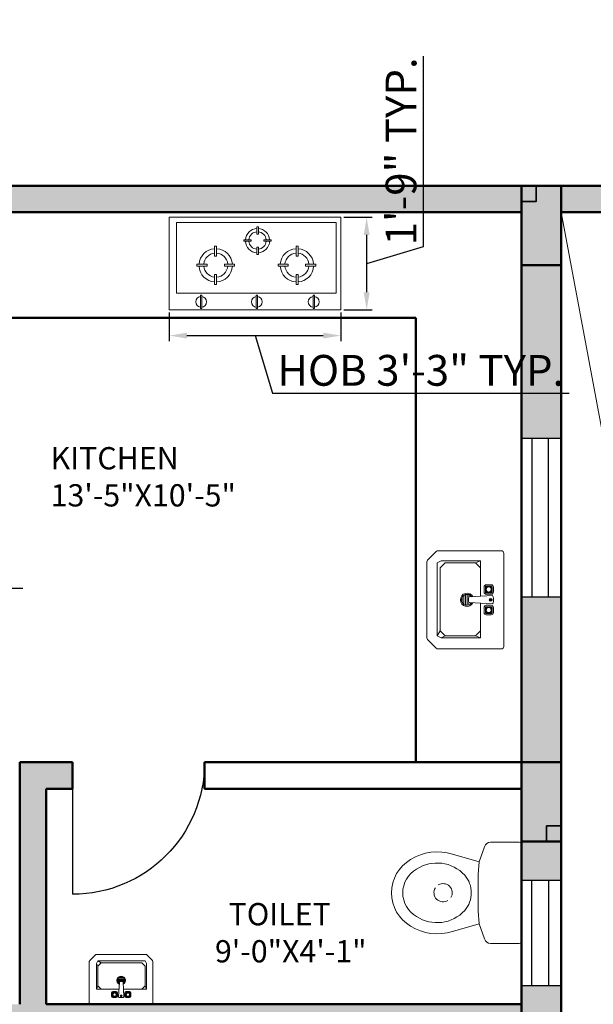
# Model space of a CAD drawing. Units: inches. Extents: x -7 to 1228, y -146 to 1091.
# Tile 25 of 88: x 433 to 563, y 307 to 531. Entities that reach past the tile are written whole.
import ezdxf

# ---------------------------------------------------------------- set-up
doc = ezdxf.new("R2010")
doc.units = ezdxf.units.IN
for name, color, linetype, lineweight in [('A-ANNO-DIMS', 2, 'Continuous', 18), ('A-AREA-IDEN', 7, 'Continuous', 18), ('A-COLS', 6, 'Continuous', 35), ('A-DOOR', 4, 'Continuous', 25), ('A-FLOR-FIXT', 8, 'Continuous', 18), ('A-FLOR-VOID', 7, 'Continuous', 18), ('A-FURN', 8, 'Continuous', 18), ('A-GLAZ', 175, 'Continuous', 25), ('A-WALL', 7, 'Continuous', 50), ('A-WALL-PATT', 251, 'Continuous', 13)]:
    doc.layers.add(name, color=color, linetype=linetype, lineweight=lineweight)
doc.styles.get("Standard").update_dxf_attribs({"font": 'arial.ttf'})
doc.dimstyles.new('ISO-25', dxfattribs={"dimtxt": 7, "dimasz": 4, "dimexe": 1.25, "dimexo": 0.625, "dimtad": 1, "dimdec": 1, "dimlunit": 3, "dimtxsty": 'Standard', "dimcen": 2.5, "dimadec": 0, "dimazin": 0, "dimtfac": 1, "dimtdec": 1, "dimtmove": 1, "dimatfit": 3, "dimfxl": 1, "dimarcsym": 0})

# ---------------------------------------------------------------- blocks, each defined once
blk = doc.blocks.new('A$C72243D80')
at = {"ltscale": 1000}
for p, q in [((0, 0), (0, 384.2)), ((0, 384.2), (712, 384.2)), ((712, 384.2), (712, 0)), ((29.5, 68.9), (29.5, 363.2)), ((29.5, 363.2), (692.7, 363.2)), ((363.5, 314.5), (363.5, 345.1)), ((363.5, 345.1), (369.5, 345.1)), ((369.5, 345.1), (369.5, 314.5)), ((692.7, 363.2), (692.7, 68.9)), ((309.4, 291), (340, 291)), ((309.4, 285), (309.4, 291)), ((340, 291), (340, 285)), ((369.5, 314.5), (363.5, 314.5)), ((392.3, 291), (392.3, 285)), ((422.9, 291), (392.3, 291)), ((422.9, 285), (422.9, 291)), ((188.1, 264.2), (188.1, 222.1)), ((196.4, 264.2), (188.1, 264.2)), ((196.4, 222.1), (196.4, 264.2)), ((340, 285), (309.4, 285)), ((363.5, 260), (363.5, 229.4)), ((369.5, 260), (363.5, 260)), ((369.5, 229.4), (369.5, 260)), ((392.3, 285), (422.9, 285)), ((525.9, 222.1), (525.9, 264.2)), ((525.9, 264.2), (534.1, 264.2)), ((534.1, 264.2), (534.1, 222.1)), ((188.1, 222.1), (196.4, 222.1)), ((363.5, 229.4), (369.5, 229.4)), ((534.1, 222.1), (525.9, 222.1)), ((114.7, 189.8), (156.8, 189.8)), ((114.7, 181.6), (114.7, 189.8)), ((156.8, 181.6), (114.7, 181.6)), ((156.8, 189.8), (156.8, 181.6)), ((228.6, 189.8), (228.6, 181.6)), ((270.7, 189.8), (228.6, 189.8)), ((228.6, 181.6), (270.7, 181.6)), ((270.7, 181.6), (270.7, 189.8)), ((451.5, 189.8), (493.6, 189.8)), ((451.5, 181.6), (451.5, 189.8)), ((493.6, 181.6), (451.5, 181.6)), ((493.6, 189.8), (493.6, 181.6)), ((565.5, 189.8), (565.5, 181.6)), ((607.6, 189.8), (565.5, 189.8)), ((565.5, 181.6), (607.6, 181.6)), ((607.6, 181.6), (607.6, 189.8)), ((188.1, 147.2), (196.4, 147.2)), ((188.1, 105.1), (188.1, 147.2)), ((196.4, 147.2), (196.4, 105.1)), ((525.9, 147.2), (525.9, 105.1)), ((534.1, 147.2), (525.9, 147.2)), ((534.1, 105.1), (534.1, 147.2)), ((196.4, 105.1), (188.1, 105.1)), ((525.9, 105.1), (534.1, 105.1)), ((692.7, 68.9), (29.5, 68.9)), ((129.6, 61.1), (129.6, 5)), ((134.4, 61.1), (129.6, 61.1)), ((134.4, 5), (134.4, 61.1)), ((360.9, 5), (360.9, 61.1)), ((360.9, 61.1), (365.7, 61.1)), ((365.7, 61.1), (365.7, 5)), ((597, 5), (597, 61.1)), ((597, 61.1), (601.8, 61.1)), ((601.8, 61.1), (601.8, 5)), ((712, 0), (0, 0)), ((129.6, 5), (134.4, 5)), ((365.7, 5), (360.9, 5)), ((601.8, 5), (597, 5))]:
    blk.add_line(p, q, dxfattribs=at)
for centre, radius, start, end in [((366.2, 287.2), 50.3, 93.0344, 175.7271), ((366.2, 287.2), 50.3, 4.2729, 86.1838), ((366.1, 287.8), 36.3, 94.0374, 175.0142), ((366.1, 287.8), 36.3, 4.9858, 84.5356), ((192.7, 184.7), 69.2, 93.8162, 175.7271), ((192.7, 184.7), 69.2, 4.2729, 86.9656), ((366.2, 287.2), 50.3, 182.5783, 266.9656), ((366.1, 287.8), 36.3, 184.5153, 265.9626), ((366.1, 287.8), 36.3, 275.4644, 355.4847), ((366.2, 287.2), 50.3, 273.8162, 357.4217), ((529.5, 184.7), 69.2, 93.0344, 175.7271), ((529.5, 184.7), 69.2, 4.2729, 86.1838), ((192.9, 185.5), 49.9, 95.4644, 175.0142), ((192.9, 185.5), 49.9, 4.9858, 85.9626), ((529.4, 185.5), 49.9, 94.0374, 175.0142), ((529.4, 185.5), 49.9, 4.9858, 84.5356), ((192.7, 184.7), 69.2, 182.5783, 266.1838), ((192.9, 185.5), 49.9, 184.5153, 264.5356), ((192.9, 185.5), 49.9, 274.0374, 355.4847), ((192.7, 184.7), 69.2, 273.0344, 357.4217), ((529.5, 184.7), 69.2, 182.5783, 266.9656), ((529.4, 185.5), 49.9, 184.5153, 265.9626), ((529.5, 184.7), 69.2, 273.8162, 357.4217), ((529.4, 185.5), 49.9, 275.4644, 355.4847), ((132.3, 33.2), 22.5, 96.7453, 263.2547), ((132.3, 33.2), 22.5, 275.4789, 84.5211), ((363.1, 33.2), 22.5, 95.4789, 264.5211), ((363.1, 33.2), 22.5, 276.7453, 83.2547), ((599.2, 33.2), 22.5, 95.4789, 264.5211), ((599.2, 33.2), 22.5, 276.7453, 83.2547)]:
    blk.add_arc(centre, radius, start, end, dxfattribs=at)
blk = doc.blocks.new('A$C4CB854FF')
for p, q in [((0, 0.3675), (0, 0.0552)), ((0.4725, 0.38), (0.0125, 0.38)), ((0.485, 0.0552), (0.485, 0.3675)), ((0.1677, 0.2932), (0.1677, 0.318)), ((0.1745, 0.2919), (0.1745, 0.3194)), ((0.1773, 0.3221), (0.2048, 0.3221)), ((0.1787, 0.329), (0.2034, 0.329)), ((0.2075, 0.3194), (0.2075, 0.2919)), ((0.2144, 0.318), (0.2144, 0.2932)), ((0.2279, 0.2104), (0.2213, 0.3235)), ((0.2337, 0.329), (0.2502, 0.329)), ((0.2625, 0.3235), (0.256, 0.2104)), ((0.2694, 0.318), (0.2694, 0.2932)), ((0.2763, 0.3194), (0.2763, 0.2919)), ((0.3065, 0.3221), (0.279, 0.3221)), ((0.3052, 0.329), (0.2804, 0.329)), ((0.3093, 0.2919), (0.3093, 0.3194)), ((0.3162, 0.2932), (0.3162, 0.318)), ((0.05, 0.265), (0.2247, 0.265)), ((0.06, 0.24), (0.05, 0.265)), ((0.05, 0.07), (0.05, 0.265)), ((0.085, 0.265), (0.06, 0.24)), ((0.2048, 0.2891), (0.1773, 0.2891)), ((0.2034, 0.2822), (0.1787, 0.2822)), ((0.2591, 0.265), (0.43, 0.265)), ((0.279, 0.2891), (0.3065, 0.2891)), ((0.2804, 0.2822), (0.3052, 0.2822)), ((0.395, 0.265), (0.42, 0.24)), ((0.42, 0.24), (0.43, 0.265)), ((0.43, 0.07), (0.43, 0.265)), ((0.06, 0.24), (0.06, 0.09)), ((0.2152, 0.1984), (0.2694, 0.1984)), ((0.2297, 0.2066), (0.2165, 0.2066)), ((0.2272, 0.2149), (0.2208, 0.2149)), ((0.2505, 0.2052), (0.2334, 0.2052)), ((0.2681, 0.2066), (0.2541, 0.2066)), ((0.2638, 0.2149), (0.2566, 0.2149)), ((0.42, 0.24), (0.42, 0.09)), ((0.2681, 0.1901), (0.2165, 0.1901)), ((0.2638, 0.1819), (0.2208, 0.1819)), ((0.2533, 0.1736), (0.2313, 0.1736)), ((0.05, 0.07), (0.06, 0.05)), ((0.06, 0.09), (0.085, 0.065)), ((0.42, 0.05), (0.06, 0.05)), ((0.085, 0.065), (0.395, 0.065)), ((0.42, 0.09), (0.395, 0.065)), ((0.395, 0.065), (0.42, 0.05)), ((0.42, 0.09), (0.43, 0.07)), ((0.43, 0.07), (0.42, 0.05)), ((0.0037, 0.0463), (0.0463, 0.0037)), ((0.4387, 0.0037), (0.4813, 0.0463)), ((0.0552, 0), (0.4298, 0))]:
    blk.add_line(p, q)
for centre, radius in [((0.191, 0.3056), 0.0165), ((0.191, 0.3056), 0.0127), ((0.2419, 0.3152), 0.00688), ((0.2419, 0.3152), 0.00344), ((0.2928, 0.3056), 0.0165), ((0.2928, 0.3056), 0.0127)]:
    blk.add_circle(centre, radius)
for centre, radius, start, end in [((0.0125, 0.3675), 0.0125, 90, 180), ((0.4725, 0.3675), 0.0125, 0, 90), ((0.1787, 0.318), 0.011, 90, 180), ((0.1787, 0.2932), 0.011, 180, 270), ((0.1773, 0.3194), 0.00275, 90, 180), ((0.2034, 0.318), 0.011, 0, 90), ((0.2034, 0.2932), 0.011, 270, 0), ((0.2048, 0.3194), 0.00275, 360, 90), ((0.2329, 0.314), 0.015, 87.1975, 140.7274), ((0.2509, 0.314), 0.015, 39.2726, 92.8025), ((0.2804, 0.318), 0.011, 90, 180), ((0.2804, 0.2932), 0.011, 180, 270), ((0.279, 0.3194), 0.00275, 90, 180), ((0.3052, 0.318), 0.011, 0, 90), ((0.3052, 0.2932), 0.011, 270, 360), ((0.3065, 0.3194), 0.00275, 360, 90), ((0.1773, 0.2919), 0.00275, 180, 270), ((0.2048, 0.2919), 0.00275, 270, 0), ((0.279, 0.2919), 0.00275, 180, 270), ((0.3065, 0.2919), 0.00275, 270, 0), ((0.2423, 0.1984), 0.033, 118.6883, 62.8686), ((0.2423, 0.1984), 0.0271, 124.7758, 57.2247), ((0.2334, 0.2107), 0.0055, 183.3274, 270), ((0.2505, 0.2107), 0.0055, 270, 356.6726), ((0.0125, 0.0552), 0.0125, 180, 225), ((0.4725, 0.0552), 0.0125, 315, 0), ((0.0552, 0.0125), 0.0125, 225, 270), ((0.4298, 0.0125), 0.0125, 270, 315)]:
    blk.add_arc(centre, radius, start, end)
blk = doc.blocks.new('A$C7B5C7CD4')
at = {"ltscale": 20}
for p, q in [((0.243, 0.625), (0.011, 0.625)), ((0.243, 0.625), (0.475, 0.625)), ((0, 0.614), (0, 0.4765)), ((0.486, 0.614), (0.486, 0.4765)), ((0.0212, 0.4467), (0.0946, 0.4214)), ((0.4648, 0.4467), (0.3914, 0.4214)), ((0.0946, 0.4214), (0.0576, 0.293)), ((0.0946, 0.4214), (0.1544, 0.4173)), ((0.3316, 0.4173), (0.1544, 0.4173)), ((0.3914, 0.4214), (0.3316, 0.4173)), ((0.3914, 0.4214), (0.4284, 0.293))]:
    blk.add_line(p, q, dxfattribs=at)
for centre, radius, start, end in [((0.011, 0.614), 0.011, 90, 180), ((0.475, 0.614), 0.011, 0, 90), ((0.0315, 0.4765), 0.0315, 180, 251), ((0.4545, 0.4765), 0.0315, 289, 0), ((0.24, 0.2602), 0.123, 88.6158, 131.7414), ((0.246, 0.2602), 0.123, 48.2586, 91.3842), ((0.2796, 0.219), 0.18, 132.4207, 213.289), ((0.2064, 0.219), 0.18, 326.711, 47.5793), ((0.2796, 0.219), 0.234, 161.5846, 212.8753), ((0.2064, 0.219), 0.234, 327.1247, 18.4154), ((0.243, 0.185), 0.131, 209.6292, 270), ((0.243, 0.185), 0.131, 270, 330.3708), ((0.243, 0.185), 0.185, 210.1745, 270), ((0.243, 0.185), 0.185, 270, 329.8255)]:
    blk.add_arc(centre, radius, start, end, dxfattribs=at)
for start, end in [(58.1785, 211.8215), (238.1785, 31.8215)]:
    blk.add_arc((0.2426, 0.2481), 0.0439, start, end)
blk = doc.blocks.new('WIN-36')
for p, q in [((0, 36), (0, 0)), ((9, 36), (0, 36)), ((2.34, 36), (2.34, 0)), ((6.14, 0), (6.14, 36)), ((9, 0), (9, 36)), ((0, 0), (9, 0)), ((2.34, 0), (6.14, 0))]:
    blk.add_line(p, q)
blk = doc.blocks.new('WIN-24')
for p, q in [((0, 0), (0, 24)), ((0, 24), (9, 24)), ((2.34, 0), (2.34, 24)), ((2.34, 24), (6.14, 24)), ((6.14, 24), (6.14, 0)), ((9, 24), (9, 0)), ((9, 0), (0, 0))]:
    blk.add_line(p, q)
blk = doc.blocks.new('DOOR-750')
blk.add_line((30, 30), (30, 0))
blk.add_arc((30, 30), 30, 180, 270)
blk = doc.blocks.new('*D34')
at = {"layer": 'A-ANNO-DIMS', "color": 0, "lineweight": -2, "transparency": 16777216}
for p, q in [((466.98, 464.2), (466.98, 457.73)), ((505.97, 464.2), (505.97, 457.73)), ((470.98, 458.98), (501.97, 458.98)), ((486.48, 458.98), (490.4, 445.92)), ((490.4, 445.92), (557.85, 445.92))]:
    blk.add_line(p, q, dxfattribs=at)
at = {"layer": 'A-ANNO-DIMS', "color": 0, "transparency": 16777216}
for points in [[(470.98, 459.64), (470.98, 458.31), (466.98, 458.98)], [(501.97, 459.64), (501.97, 458.31), (505.97, 458.98)]]:
    blk.add_solid(points, dxfattribs=at)
at = {"layer": 'Defpoints', "color": 0, "transparency": 16777216}
for p in [(466.98, 464.83), (505.97, 464.83), (505.97, 458.98)]:
    blk.add_point(p, dxfattribs=at)
at = {"layer": 'A-ANNO-DIMS', "color": 0, "transparency": 16777216, "insert": (524.12, 450.17), "char_height": 7, "attachment_point": 5}
blk.add_mtext('HOB 3\'-3" TYP.', dxfattribs=at)
blk = doc.blocks.new('*D35')
at = {"layer": 'A-ANNO-DIMS', "color": 0, "lineweight": -2, "transparency": 16777216}
for p, q in [((524.73, 479.22), (524.73, 522.48)), ((506.6, 485.86), (513.07, 485.86)), ((511.82, 468.83), (511.82, 481.86)), ((511.82, 475.34), (524.73, 479.22)), ((506.6, 464.83), (513.07, 464.83))]:
    blk.add_line(p, q, dxfattribs=at)
at = {"layer": 'A-ANNO-DIMS', "color": 0, "transparency": 16777216}
for points in [[(511.15, 481.86), (512.49, 481.86), (511.82, 485.86)], [(511.15, 468.83), (512.49, 468.83), (511.82, 464.83)]]:
    blk.add_solid(points, dxfattribs=at)
at = {"layer": 'Defpoints', "color": 0, "transparency": 16777216}
for p in [(505.97, 485.86), (511.82, 485.86), (505.97, 464.83)]:
    blk.add_point(p, dxfattribs=at)
at = {"layer": 'A-ANNO-DIMS', "color": 0, "transparency": 16777216, "insert": (520.53, 500.85), "char_height": 7, "attachment_point": 5, "rotation": 90}
blk.add_mtext('1\'-9" TYP.', dxfattribs=at)
blk = doc.blocks.new('*D40')
at = {"layer": 'A-ANNO-DIMS', "color": 0, "lineweight": -2, "transparency": 16777216}
for p, q in [((301.32, 424.02), (301.32, 413.35)), ((368.31, 424.02), (368.31, 413.35)), ((305.32, 414.6), (364.31, 414.6)), ((334.82, 414.6), (338.73, 401.55)), ((338.73, 401.55), (433.69, 401.55))]:
    blk.add_line(p, q, dxfattribs=at)
at = {"layer": 'A-ANNO-DIMS', "color": 0, "transparency": 16777216}
for points in [[(305.32, 415.26), (305.32, 413.93), (301.32, 414.6)], [(364.31, 415.26), (364.31, 413.93), (368.31, 414.6)]]:
    blk.add_solid(points, dxfattribs=at)
at = {"layer": 'Defpoints', "color": 0, "transparency": 16777216}
for p in [(301.32, 424.65), (368.31, 424.65), (368.31, 414.6)]:
    blk.add_point(p, dxfattribs=at)
at = {"layer": 'A-ANNO-DIMS', "color": 0, "transparency": 16777216, "insert": (386.21, 405.79), "char_height": 7, "attachment_point": 5}
blk.add_mtext('SOFA SET 5\'-7" TYP.', dxfattribs=at)

msp = doc.modelspace()

# ---------------------------------------------------------------- hatches: boundary and pattern name
at = {"layer": 'A-COLS'}
h = msp.add_hatch(color=256, dxfattribs=at)
h.dxf.hatch_style = 1
h.paths.add_polyline_path([(547, 475), (556, 475), (556, 493), (550.29, 493), (550.29, 489.45), (547, 489.45)])
h = msp.add_hatch(color=256, dxfattribs=at)
h.dxf.hatch_style = 1
h.paths.add_polyline_path([(550.29, 489.45), (550.29, 493), (547, 493), (547, 489.45)])
h = msp.add_hatch(color=256, dxfattribs=at)
h.dxf.hatch_style = 1
h.paths.add_polyline_path([(556, 362), (547, 362), (547, 344), (552.71, 344), (552.71, 347.55), (556, 347.55)])
h = msp.add_hatch(color=256, dxfattribs=at)
h.dxf.hatch_style = 1
h.paths.add_polyline_path([(552.71, 347.55), (552.71, 344), (556, 344), (556, 347.55)])
at = {"layer": 'A-WALL-PATT'}
h = msp.add_hatch(color=256, dxfattribs=at)
h.dxf.hatch_style = 1
h.paths.add_polyline_path([(69, 568), (60, 568), (60, 493), (63.29, 493), (69, 493)])
h.paths.add_polyline_path([(69, 662.41), (60, 662.41), (60, 586), (69, 586)], flags=17)
h.paths.add_polyline_path([(69, 723), (184, 723), (184, 734), (179, 734), (179, 728), (69, 728), (69, 741.62), (60, 741.62), (60, 698.41), (69, 698.41)], flags=17)
h.paths.add_polyline_path([(69, 782), (231, 782), (231, 728), (231, 723), (231, 586), (236, 586), (236, 787), (69, 787), (69, 800.13), (60, 800.13), (60, 765.62), (69, 765.62)])
h.paths.add_polyline_path([(184, 842), (189, 842), (189, 848), (173, 848), (173, 842), (179, 842), (179, 787), (184, 787)])
h.paths.add_polyline_path([(118.22, 69), (69, 69), (69, 60), (118.22, 60)])
h.paths.add_polyline_path([(227, 69), (154.22, 69), (154.22, 60), (227, 60)])
h.paths.add_polyline_path([(236, 60), (232.71, 60), (227, 60), (227, 36), (236, 36)])
h.paths.add_polyline_path([(389, 60), (380, 60), (380, 36), (389, 36)])
h.paths.add_polyline_path([(384, 181), (380, 181), (380, 115), (380, 78), (384, 78)])
h.paths.add_polyline_path([(380, 115), (334.55, 115), (334.55, 109), (380, 109)])
h.paths.add_polyline_path([(274.55, 115), (236, 115), (236, 201), (232.71, 201), (231, 201), (231, 78), (236, 78), (236, 109), (274.55, 109)])
h.paths.add_polyline_path([(69, 123), (60, 123), (60, 78), (69, 78)])
h.paths.add_polyline_path([(69, 201), (60, 201), (60, 159), (69, 159)])
h.paths.add_polyline_path([(143, 219), (69, 219), (69, 213), (143, 213)], flags=17)
h.paths.add_polyline_path([(189, 219), (184, 219), (184, 274), (231, 274), (231, 219), (236, 219), (236, 279), (184, 279), (184, 297), (179, 297), (179, 279), (69, 279), (69, 290.91), (60, 290.91), (60, 262.18), (69, 262.18), (69, 274), (179, 274), (179, 219), (173, 219), (173, 213), (189, 213)])
h.paths.add_polyline_path([(69, 238.18), (60, 238.18), (60, 219), (69, 219)], flags=17)
h.paths.add_polyline_path([(69, 333), (60, 333), (60, 314.91), (69, 314.91), (69, 316.96)])
h.paths.add_polyline_path([(190, 338), (184, 338), (69, 338), (69, 333), (179, 333), (179, 327), (184, 327), (184, 333.02), (190, 333.05)])
h.paths.add_polyline_path([(69, 386.81), (60, 386.81), (60, 351), (69, 351)])
h.paths.add_polyline_path([(69, 475), (60, 475), (60, 422.81), (69, 422.81)])
h.paths.add_polyline_path([(236, 475), (231, 475), (231, 351.24), (236, 351.24)])
h.paths.add_polyline_path([(384, 475), (380, 475), (380, 362), (384, 362)])
h.paths.add_polyline_path([(547, 307), (439, 307), (439, 356), (445, 356), (445, 362), (433, 362), (433, 307), (380, 307), (380, 244), (380, 241), (384, 241), (384, 301), (433, 301), (433, 277), (439, 277), (439, 301), (547, 301)])
h.paths.add_polyline_path([(547, 241), (439, 241), (439, 247), (433, 247), (433, 235), (547, 235)])
h.paths.add_polyline_path([(450, 69), (440.29, 69), (424.89, 69), (389, 69), (389, 60), (450, 60)])
h.paths.add_polyline_path([(547, 69), (486, 69), (486, 60), (547, 60)])
h.paths.add_polyline_path([(556, 148.27), (547, 148.27), (547, 78), (556, 78)])
h.paths.add_polyline_path([(556, 223), (547, 223), (547, 195), (547, 184.27), (556, 184.27)])
h.paths.add_polyline_path([(556, 311.19), (547, 311.19), (547, 273.08), (556, 273.08)])
h.paths.add_polyline_path([(556, 344), (552.71, 344), (547, 344), (547, 335.19), (556, 335.19)])
h.paths.add_polyline_path([(556, 249.08), (547, 249.08), (547, 241), (556, 241)])
h.paths.add_polyline_path([(547, 362), (475, 362), (475, 356), (547, 356)], flags=0)
h.paths.add_polyline_path([(556, 399.62), (547, 399.62), (547, 362), (556, 362)])
h.paths.add_polyline_path([(556, 475), (547, 475), (547, 435.62), (556, 435.62)])
h.paths.add_polyline_path([(547, 493), (389, 493), (389, 487), (547, 487)])
h.paths.add_polyline_path([(380, 493), (278, 493), (278, 487), (380, 487)])
h.paths.add_polyline_path([(227, 493), (69, 493), (69, 487), (227, 487)])
h.paths.add_polyline_path([(643, 122.44), (634, 122.44), (634, 78), (643, 78)])
h.paths.add_polyline_path([(702.5, 69), (692.79, 69), (677.39, 69), (643, 69), (643, 60), (702.5, 60)])
h.paths.add_polyline_path([(798, 69), (738.5, 69), (738.5, 60), (798, 60)])
h.paths.add_polyline_path([(807, 60), (803.71, 60), (798, 60), (798, 36), (807, 36)])
h.paths.add_polyline_path([(807, 109), (846.75, 109), (846.75, 115), (807, 115), (807, 159), (802, 159), (802, 78), (807, 78)])
h.paths.add_polyline_path([(807, 201), (802, 201), (802, 195), (807, 195)])
h.paths.add_polyline_path([(643, 201), (634, 201), (634, 158.44), (643, 158.44)])
h.paths.add_polyline_path([(756, 225), (751, 225), (751, 219), (643, 219), (643, 213), (756, 213)])
h.paths.add_polyline_path([(643, 240.85), (634, 240.85), (634, 219), (643, 219)])
h.paths.add_polyline_path([(643, 274), (643, 288.63), (634, 288.63), (634, 264.85), (643, 264.85)])
h.paths.add_polyline_path([(802, 279), (756, 279), (756, 297), (751, 297), (751, 279), (643, 279), (643, 274), (751, 274), (751, 255), (756, 255), (756, 274), (802, 274)])
h.paths.add_polyline_path([(807, 333), (803.71, 333), (802, 333), (802, 279), (802, 274), (802, 219), (807, 219)])
h.paths.add_polyline_path([(956, 182), (951, 182), (951, 115), (906.75, 115), (906.75, 109), (951, 109), (951, 78), (956, 78)])
h.paths.add_polyline_path([(960, 60), (951, 60), (951, 36), (960, 36)])
h.paths.add_polyline_path([(1021, 69), (1005.78, 69), (960, 69), (960, 60), (1021, 60)])
h.paths.add_polyline_path([(956, 224), (951, 224), (951, 218), (956, 218)])
h.paths.add_polyline_path([(956, 302), (1004, 302), (1004, 278), (1010, 278), (1010, 302), (1118, 302), (1118, 290.81), (1127, 290.81), (1127, 326.97), (1118, 326.97), (1118, 320.97), (1118, 307), (1010, 307), (1010, 356), (1016, 356), (1016, 362), (1004, 362), (1004, 307), (951, 307), (951, 244), (951, 242), (954.29, 242), (956, 242)])
h.paths.add_polyline_path([(643, 333), (634, 333), (634, 312.63), (643, 312.63), (643, 316.96)])
h.paths.add_polyline_path([(756, 338), (643, 338), (643, 333), (751, 333), (751, 327), (756, 327)])
h.paths.add_polyline_path([(643, 388), (634, 388), (634, 351), (643, 351)])
h.paths.add_polyline_path([(807, 357), (802, 357), (802, 351), (807, 351)])
h.paths.add_polyline_path([(807, 475), (802, 475), (802, 393), (807, 393)])
h.paths.add_polyline_path([(643, 475), (634, 475), (634, 424), (643, 424)])
h.paths.add_polyline_path([(798, 493), (643, 493), (643, 487), (798, 487)])
h.paths.add_polyline_path([(634, 493), (556, 493), (556, 487), (634, 487)])
h.paths.add_polyline_path([(813, 493), (807, 493), (807, 487), (813, 487)])
h.paths.add_polyline_path([(951, 493), (849, 493), (849, 487), (951, 487)])
h.paths.add_polyline_path([(956, 484), (951, 484), (951, 374), (956, 374)])
h.paths.add_polyline_path([(1109, 493), (969, 493), (969, 487), (1109, 487)])
h.paths.add_polyline_path([(1127, 484), (1118, 484), (1118, 450.64), (1127, 450.64)])
h.paths.add_polyline_path([(1127, 414.64), (1118, 414.64), (1118, 365), (1127, 365)])
h.paths.add_polyline_path([(1109, 362), (1046, 362), (1046, 356), (1109, 356)], flags=17)
h.paths.add_polyline_path([(1127, 356), (1123.45, 356), (1118, 356), (1118, 350.97), (1127, 350.97)], flags=0)
h.paths.add_polyline_path([(1127, 266.81), (1118, 266.81), (1118, 262.36), (1118, 242), (1127, 242)], flags=17)
h.paths.add_polyline_path([(1118, 242), (1010, 242), (1010, 248), (1004, 248), (1004, 237), (1118, 237)])
h.paths.add_polyline_path([(1127, 224), (1118, 224), (1118, 170), (1127, 170)])
h.paths.add_polyline_path([(1127, 134), (1118, 134), (1118, 78), (1127, 78)])
h.paths.add_polyline_path([(1118, 69), (1057, 69), (1057, 60), (1118, 60)])
h.paths.add_polyline_path([(227, 571.55), (227, 574), (69, 574), (69, 568), (227, 568)])
h.paths.add_polyline_path([(380, 571.55), (380, 574), (278, 574), (278, 568), (380, 568)])
h.paths.add_polyline_path([(242, 574), (236, 574), (236, 568), (242, 568)])
h.paths.add_polyline_path([(547, 571.55), (547, 574), (389, 574), (389, 568), (547, 568)])
h.paths.add_polyline_path([(384, 733), (380, 733), (380, 586), (384, 586)])
h.paths.add_polyline_path([(556, 646), (634, 646), (634, 655), (547, 655), (547, 586), (556, 586)])
h.paths.add_polyline_path([(634, 574), (556, 574), (556, 568), (634, 568)])
h.paths.add_polyline_path([(643, 655), (634, 655), (634, 586), (643, 586)])
h.paths.add_polyline_path([(798, 574), (643, 574), (643, 568), (798, 568)])
h.paths.add_polyline_path([(643, 663.85), (634, 663.85), (634, 655), (643, 655)])
h.paths.add_polyline_path([(556, 676.97), (547, 676.97), (547, 655), (556, 655)])
h.paths.add_polyline_path([(556, 733), (547, 733), (547, 712.97), (556, 712.97)])
h.paths.add_polyline_path([(643, 710), (634, 710), (634, 699.85), (643, 699.85)])
h.paths.add_polyline_path([(807, 668), (802, 668), (802, 586), (807, 586)])
h.paths.add_polyline_path([(951, 574), (849, 574), (849, 568), (951, 568)])
h.paths.add_polyline_path([(956, 691), (951, 691), (951, 577), (956, 577)])
h.paths.add_polyline_path([(1109, 574), (969, 574), (969, 568), (1109, 568)])
h.paths.add_polyline_path([(1127, 643.4), (1118, 643.4), (1118, 577), (1127, 577)])
h.paths.add_polyline_path([(1127, 568), (1123.45, 568), (1118, 568), (1118, 493), (1127, 493)])
h.paths.add_polyline_path([(1127, 733), (1118, 733), (1118, 679.4), (1127, 679.4)])
h.paths.add_polyline_path([(1127, 777.35), (1118, 777.35), (1118, 770.04), (1118, 751), (1127, 751)], flags=17)
h.paths.add_polyline_path([(1118, 751), (1010, 751), (1010, 757), (1004, 757), (1004, 745), (1118, 745)])
h.paths.add_polyline_path([(956, 811), (1004, 811), (1004, 787), (1010, 787), (1010, 811), (1017.87, 811), (1017.87, 811.63, -0.414214), (1018.25, 812), (1031.98, 812, -0.414214), (1032.35, 811.63), (1032.35, 811), (1118, 811), (1118, 801.35), (1127, 801.35), (1127, 834.69), (1118, 834.69), (1118, 830.24), (1118, 817), (1010, 817), (1010, 866), (1016, 866), (1016, 872), (1004, 872), (1004, 817), (956, 817), (956, 866), (951, 866), (951, 751), (954.29, 751), (956, 751)])
h.paths.add_polyline_path([(1118, 872), (1046, 872), (1046, 866), (1118, 866)], flags=17)
h.paths.add_polyline_path([(1127, 924.71), (1118, 924.71), (1118, 884), (1127, 884)])
h.paths.add_polyline_path([(1127, 866), (1123.71, 866), (1118, 866), (1118, 858.69), (1127, 858.69)], flags=17)
h.paths.add_polyline_path([(956, 983), (951, 983), (951, 952), (807, 952), (807, 983), (802, 983), (802, 902), (807, 902), (807, 946), (951, 946), (951, 884), (956, 884)])
h.paths.add_polyline_path([(807, 842), (802, 842), (802, 787), (756, 787), (756, 806), (751, 806), (751, 787), (643, 787), (643, 782), (751, 782), (751, 764), (756, 764), (756, 782), (802, 782), (802, 728), (807, 728)])
h.paths.add_polyline_path([(756, 848), (643, 848), (643, 842), (751, 842), (751, 836), (756, 836)])
h.paths.add_polyline_path([(756, 734), (751, 734), (751, 728), (643, 728), (643, 723), (756, 723)])
h.paths.add_polyline_path([(643, 749.79), (634, 749.79), (634, 728), (637.29, 728), (643, 728)])
h.paths.add_polyline_path([(643, 805.41), (634, 805.41), (634, 773.79), (643, 773.79)])
h.paths.add_polyline_path([(643, 896.66), (634, 896.66), (634, 860), (637.29, 860), (643, 860)])
h.paths.add_polyline_path([(643, 842), (634, 842), (634, 829.41), (643, 829.41)])
h.paths.add_polyline_path([(643, 983), (634, 983), (634, 932.66), (643, 932.66)])
h.paths.add_polyline_path([(1127, 983), (1118, 983), (1118, 960.71), (1127, 960.71)])
h.paths.add_polyline_path([(1118, 1001), (1077.53, 1001), (1077.53, 992), (1118, 992)])
h.paths.add_polyline_path([(1041.53, 1001), (960, 1001), (960, 992), (1041.53, 992)])
h.paths.add_polyline_path([(960, 1025), (951, 1025), (951, 1001), (954.29, 1001), (960, 1001)])
h.paths.add_polyline_path([(807, 1025), (798, 1025), (798, 1001), (807, 1001)])
h.paths.add_polyline_path([(798, 1001), (738.5, 1001), (738.5, 992), (798, 992)])
h.paths.add_polyline_path([(702.5, 1001), (643, 1001), (643, 992), (702.5, 992)])
h.paths.add_polyline_path([(547, 1001), (499.11, 1001), (499.11, 992), (547, 992)])
h.paths.add_polyline_path([(463.11, 1001), (389, 1001), (389, 992), (463.11, 992)])
h.paths.add_polyline_path([(389, 1025), (380, 1025), (380, 1022), (380, 1001), (383.29, 1001), (389, 1001)])
h.paths.add_polyline_path([(236, 1025), (227, 1025), (227, 1001), (236, 1001)])
h.paths.add_polyline_path([(236, 983), (231, 983), (231, 860), (236, 860)])
h.paths.add_polyline_path([(274.55, 952), (236, 952), (236, 946), (274.55, 946)])
h.paths.add_polyline_path([(380, 952), (334.55, 952), (334.55, 946), (380, 946)])
h.paths.add_polyline_path([(384, 983), (380, 983), (380, 884), (383.29, 884), (384, 884)])
h.paths.add_polyline_path([(227, 1001), (155.01, 1001), (155.01, 992), (162.87, 992), (227, 992)])
h.paths.add_polyline_path([(119.01, 1001), (69, 1001), (69, 992), (119.01, 992)])
h.paths.add_polyline_path([(69, 983), (60, 983), (60, 922.99), (69, 922.99)])
h.paths.add_polyline_path([(69, 886.99), (60, 886.99), (60, 860), (63.29, 860), (69, 860)])
h.paths.add_polyline_path([(143, 848), (69, 848), (69, 842), (143, 842)])

# ---------------------------------------------------------------- linework, layer by layer
at = {"layer": 'A-COLS'}
for points in [[(547, 493), (550.29, 493), (550.29, 489.45), (547, 489.45)], [(556, 344), (552.71, 344), (552.71, 347.55), (556, 347.55)]]:
    msp.add_lwpolyline(points, close=True, dxfattribs=at)
at = {"layer": 'A-FLOR-VOID'}
msp.add_line((556, 487), (634, 69), dxfattribs=at)
at = {"layer": 'A-WALL'}
for p, q in [((547, 493), (384, 493)), ((547, 493), (547, 60)), ((547, 493), (556, 493)), ((547, 475), (547, 493)), ((556, 493), (556, 60)), ((813, 493), (556, 493)), ((556, 493), (556, 475)), ((547, 487), (384, 487)), ((547, 316), (547, 487)), ((813, 487), (556, 487)), ((556, 415), (556, 487)), ((556, 475), (547, 475)), ((523, 463), (384, 463)), ((523, 362), (523, 463)), ((556, 60), (556, 406)), ((433, 307), (433, 362)), ((445, 362), (433, 362)), ((445, 356), (445, 362)), ((547, 362), (475, 362)), ((475, 356), (475, 362)), ((547, 344), (547, 362)), ((547, 362), (556, 362)), ((556, 362), (556, 344)), ((439, 307), (439, 356)), ((445, 356), (439, 356)), ((547, 356), (475, 356)), ((556, 344), (547, 344)), ((547, 250), (547, 310)), ((547, 307), (439, 307))]:
    msp.add_line(p, q, dxfattribs=at)

# ---------------------------------------------------------------- block references
at = {"layer": 'A-DOOR', "extrusion": (0, 0, -1), "zscale": -1}
msp.add_blockref('DOOR-750', (-475, 332), dxfattribs=at)
at = {"layer": 'A-FLOR-FIXT', "xscale": 47.26153857112405, "yscale": 47.26153857112405, "zscale": 47.26153857112405, "rotation": 270}
msp.add_blockref('A$C7B5C7CD4', (517.46, 343.82), dxfattribs=at)
at = {"layer": 'A-FURN', "xscale": 0.0547573419986423, "yscale": 0.0547573419986423, "zscale": 0.0547573419986423}
msp.add_blockref('A$C72243D80', (466.98, 464.83), dxfattribs=at)
at = {"layer": 'A-FURN'}
for p, xscale, yscale, zscale, rotation in [((525.5, 410.07), 45.99182974636398, 45.99182974636398, 45.99182974636398, 270), ((463.28, 318.34), 29.84864686937646, 29.84864686937646, 29.84864686937646, 180)]:
    msp.add_blockref('A$C4CB854FF', p, dxfattribs=dict(at, xscale=xscale, yscale=yscale, zscale=zscale, rotation=rotation))
at = {"layer": 'A-GLAZ'}
for name, p in [('WIN-36', (547, 399.62)), ('WIN-24', (547, 311.19))]:
    msp.add_blockref(name, p, dxfattribs=at)

# ---------------------------------------------------------------- texts
at = {"layer": 'A-AREA-IDEN', "char_height": 5.0568, "attachment_point": 1}
for s, insert in [(' KITCHEN\\P 13\'-5"X10\'-5"', (438.48, 433.63)), ('  TOILET\\P9\'-0"X4\'-1"', (477.36, 330.01))]:
    msp.add_mtext_dynamic_manual_height_columns(s, width=137.2821, gutter_width=25.28, heights=[0], dxfattribs=dict(at, insert=insert))

# ---------------------------------------------------------------- dimensions: what is measured, and where the dimension line sits
at = {"layer": 'A-ANNO-DIMS'}
dim = msp.add_linear_dim(base=(511.82, 485.86), p1=(505.97, 464.83), p2=(505.97, 485.86), angle=90, text='<> TYP.', dimstyle='ISO-25', override={"dimdec": 1, "dimlfac": 1, "dimrnd": 0, "dimzin": 1, "dimdsep": 46, "dimlunit": 4, "dimfrac": 2}, dxfattribs=at)
dim.commit()
dim.dimension.update_dxf_attribs({"geometry": '*D35', "text_midpoint": (520.53, 479.84)})
for base, p1, p2, text, picture, middle in [((505.97, 458.98), (466.98, 464.83), (505.97, 464.83), 'HOB <> TYP.', '*D34', (491.02, 450.17)), ((368.31, 414.6), (301.32, 424.65), (368.31, 424.65), 'SOFA SET <> TYP.', '*D40', (339.36, 405.79))]:
    dim = msp.add_linear_dim(base=base, p1=p1, p2=p2, text=text, dimstyle='ISO-25', override={"dimdec": 1, "dimlfac": 1, "dimrnd": 0, "dimzin": 1, "dimdsep": 46, "dimlunit": 4, "dimfrac": 2}, dxfattribs=at)
    dim.commit()
    dim.dimension.update_dxf_attribs({"geometry": picture, "text_midpoint": middle})

doc.saveas('drawing.dxf')
